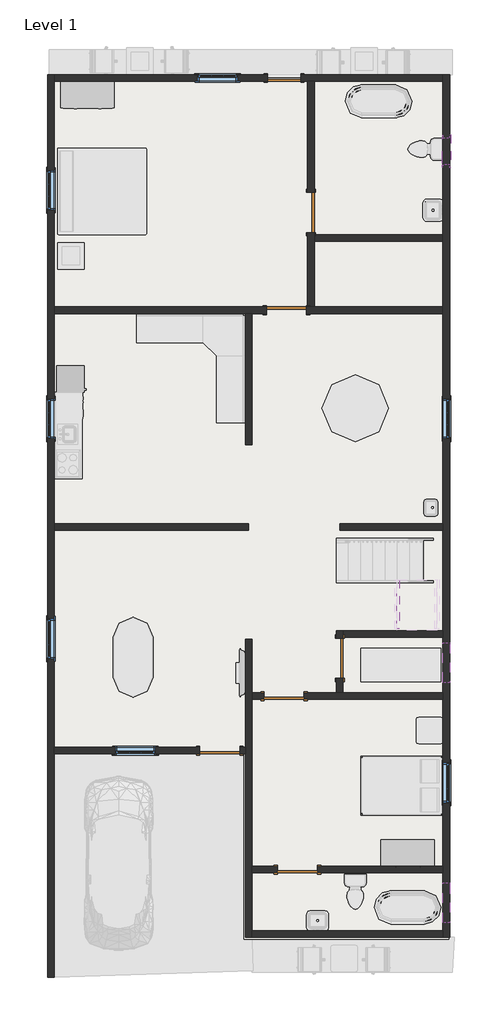
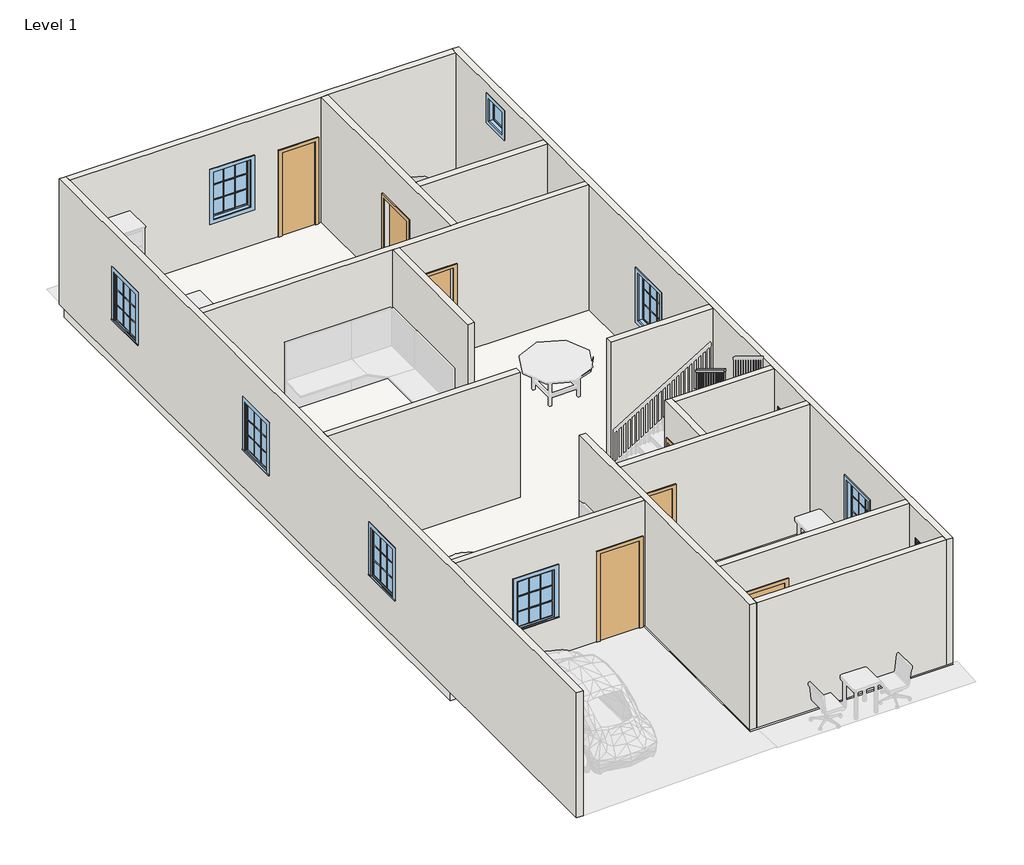
# One storey, part 1 of 2: 16 walls, 10 windows, 7 doors, 1 railing, 1 slab.
"""IFC4 building model written with IfcOpenShell, lengths in millimetres."""

from ifc_helpers import new_model, si_unit, frame, origin, origin_with_axes, place, context, project, spatial, polyline, outline, extrude, faceted_brep, transform, mapped, element, save
from components import door_255cab33, door_16372e1c, door_686f89d2, window_5c190c7e, window_fef7ae9c, window_3d781103

model = new_model("IFC4")

# Units and contexts
model_context = context("Model", 3, world=origin())
ifc_project = project(units=[si_unit("LENGTHUNIT", "METRE", prefix="MILLI")], contexts=[model_context])

# Site, building, storey
site = spatial("IfcSite", under=ifc_project)
building = spatial("IfcBuilding", under=site)
storey = spatial("IfcBuildingStorey", under=building, Name="Level 1", Elevation=0.0)

# Doors
placement = place(None, origin())
door_shape = door_255cab33(model_context)
element("IfcDoor", 1, ObjectType="Single-Flush : 30\" x 80\"", at=placement, inside=storey, context=model_context, shape_type="MappedRepresentation", body=[
    mapped(door_shape, transform((-7141.5873398, 12389.5549175, 0.0), x_axis=(1.0, 0.0, 0.0), y_axis=(0.0, 1.0, 0.0), z_axis=(0.0, 0.0, 1.0))),
])
door_2_shape = door_16372e1c(model_context)
element("IfcDoor", 2, ObjectType="Single-Flush : 36\" x 84\"", at=placement, inside=storey, context=model_context, shape_type="MappedRepresentation", body=[
    mapped(door_2_shape, transform((-7090.7873398, 7080.9549175, 0.0), x_axis=(1.0, 0.0, 0.0), y_axis=(0.0, 1.0, 0.0), z_axis=(0.0, 0.0, 1.0))),
])
element("IfcDoor", 3, ObjectType="Single-Flush : 36\" x 84\"", at=placement, inside=storey, context=model_context, shape_type="MappedRepresentation", body=[
    mapped(door_2_shape, transform((-6531.9873398, 9316.1549175, 0.0), x_axis=(0.0, -1.0, 0.0), y_axis=(1.0, 0.0, 0.0), z_axis=(0.0, 0.0, 1.0))),
])
element("IfcDoor", 4, ObjectType="Single-Flush : 36\" x 84\"", at=placement, inside=storey, context=model_context, shape_type="MappedRepresentation", body=[
    mapped(door_2_shape, transform((-7141.5873398, -1732.8450825, 0.0), x_axis=(-1.0, 0.0, 0.0), y_axis=(0.0, -1.0, 0.0), z_axis=(0.0, 0.0, 1.0))),
])
element("IfcDoor", 5, ObjectType="Single-Flush : 36\" x 84\"", at=placement, inside=storey, context=model_context, shape_type="MappedRepresentation", body=[
    mapped(door_2_shape, transform((-6836.7873398, -5695.2450825, 0.0), x_axis=(-1.0, 0.0, 0.0), y_axis=(0.0, -1.0, 0.0), z_axis=(0.0, 0.0, 1.0))),
])
door_3_shape = door_686f89d2(model_context)
element("IfcDoor", 6, ObjectType="Single-Flush : 36\" x 84\"", at=placement, inside=storey, context=model_context, shape_type="MappedRepresentation", body=[
    mapped(door_3_shape, transform((-8614.7873398, -2977.4450825, 0.0), x_axis=(1.0, 0.0, 0.0), y_axis=(0.0, 1.0, 0.0), z_axis=(0.0, 0.0, 1.0))),
])
element("IfcDoor", 7, ObjectType="Single-Flush : 36\" x 84\"", at=placement, inside=storey, context=model_context, shape_type="MappedRepresentation", body=[
    mapped(door_3_shape, transform((-5871.5873398, -869.2450825, 0.0), x_axis=(0.0, 1.0, 0.0), y_axis=(-1.0, 0.0, 0.0), z_axis=(0.0, 0.0, 1.0))),
])

# Railing
element("IfcRailing", 8, ObjectType="Handrail - Rectangular", at=placement, inside=storey, context=model_context, shape_type="SweptSolid", body=[
    extrude(outline(polyline([(923.5061342, 2607.7333333), (923.5061342, 2548.3318731), (-194.0938658, 3225.6652064), (-194.0938658, 3285.0666667), (923.5061342, 2607.7333333)])), frame((-4563.8448749, 0.0, 0.0), z_axis=(1.0, 0.0, 0.0), x_axis=(0.0, 1.0, 0.0)), (0.0, 0.0, 1.0), 50.8),
    extrude(outline(polyline([(831.4311342, 2604.1349034), (831.4311342, 1693.3333333), (812.3811342, 1693.3333333), (812.3811342, 2615.6803579), (831.4311342, 2604.1349034)])), frame((-4547.9698749, 0.0, 0.0), z_axis=(1.0, 0.0, 0.0), x_axis=(0.0, 1.0, 0.0)), (0.0, 0.0, 1.0), 19.05),
    extrude(outline(polyline([(729.8311342, 2665.710661), (729.8311342, 1693.3333333), (710.7811342, 1693.3333333), (710.7811342, 2677.2561155), (729.8311342, 2665.710661)])), frame((-4547.9698749, 0.0, 0.0), z_axis=(1.0, 0.0, 0.0), x_axis=(0.0, 1.0, 0.0)), (0.0, 0.0, 1.0), 19.05),
    extrude(outline(polyline([(628.2311342, 2727.2864185), (628.2311342, 1862.6666667), (609.1811342, 1862.6666667), (609.1811342, 2738.8318731), (628.2311342, 2727.2864185)])), frame((-4547.9698749, 0.0, 0.0), z_axis=(1.0, 0.0, 0.0), x_axis=(0.0, 1.0, 0.0)), (0.0, 0.0, 1.0), 19.05),
    extrude(outline(polyline([(526.6311342, 2788.8621761), (526.6311342, 1862.6666667), (507.5811342, 1862.6666667), (507.5811342, 2800.4076307), (526.6311342, 2788.8621761)])), frame((-4547.9698749, 0.0, 0.0), z_axis=(1.0, 0.0, 0.0), x_axis=(0.0, 1.0, 0.0)), (0.0, 0.0, 1.0), 19.05),
    extrude(outline(polyline([(425.0311342, 2850.4379337), (425.0311342, 1862.6666667), (405.9811342, 1862.6666667), (405.9811342, 2861.9833882), (425.0311342, 2850.4379337)])), frame((-4547.9698749, 0.0, 0.0), z_axis=(1.0, 0.0, 0.0), x_axis=(0.0, 1.0, 0.0)), (0.0, 0.0, 1.0), 19.05),
    extrude(outline(polyline([(323.4311342, 2912.0136913), (323.4311342, 2032.0), (304.3811342, 2032.0), (304.3811342, 2923.5591458), (323.4311342, 2912.0136913)])), frame((-4547.9698749, 0.0, 0.0), z_axis=(1.0, 0.0, 0.0), x_axis=(0.0, 1.0, 0.0)), (0.0, 0.0, 1.0), 19.05),
    extrude(outline(polyline([(221.8311342, 2973.5894488), (221.8311342, 2032.0), (202.7811342, 2032.0), (202.7811342, 2985.1349034), (221.8311342, 2973.5894488)])), frame((-4547.9698749, 0.0, 0.0), z_axis=(1.0, 0.0, 0.0), x_axis=(0.0, 1.0, 0.0)), (0.0, 0.0, 1.0), 19.05),
    extrude(outline(polyline([(120.2311342, 3035.1652064), (120.2311342, 2032.0), (101.1811342, 2032.0), (101.1811342, 3046.710661), (120.2311342, 3035.1652064)])), frame((-4547.9698749, 0.0, 0.0), z_axis=(1.0, 0.0, 0.0), x_axis=(0.0, 1.0, 0.0)), (0.0, 0.0, 1.0), 19.05),
    extrude(outline(polyline([(18.6311342, 3096.740964), (18.6311342, 2201.3333333), (-0.4188658, 2201.3333333), (-0.4188658, 3108.2864185), (18.6311342, 3096.740964)])), frame((-4547.9698749, 0.0, 0.0), z_axis=(1.0, 0.0, 0.0), x_axis=(0.0, 1.0, 0.0)), (0.0, 0.0, 1.0), 19.05),
    extrude(outline(polyline([(-82.9688658, 3158.3167216), (-82.9688658, 2201.3333333), (-102.0188658, 2201.3333333), (-102.0188658, 3169.8621761), (-82.9688658, 3158.3167216)])), frame((-4547.9698749, 0.0, 0.0), z_axis=(1.0, 0.0, 0.0), x_axis=(0.0, 1.0, 0.0)), (0.0, 0.0, 1.0), 19.05),
    extrude(outline(polyline([(923.5061342, 2548.3318731), (923.5061342, 1693.3333333), (904.4561342, 1693.3333333), (904.4561342, 2559.8773276), (923.5061342, 2548.3318731)])), frame((-4547.9698749, 0.0, 0.0), z_axis=(1.0, 0.0, 0.0), x_axis=(0.0, 1.0, 0.0)), (0.0, 0.0, 1.0), 19.05),
    extrude(outline(polyline([(-175.0438658, 3214.1197519), (-175.0438658, 2201.3333333), (-194.0938658, 2201.3333333), (-194.0938658, 3225.6652064), (-175.0438658, 3214.1197519)])), frame((-4547.9698749, 0.0, 0.0), z_axis=(1.0, 0.0, 0.0), x_axis=(0.0, 1.0, 0.0)), (0.0, 0.0, 1.0), 19.05),
])

# Slab
element("IfcSlab", 9, ObjectType="Generic - 12\"", at=placement, inside=storey, context=model_context, shape_type="SweptSolid", body=[
    extrude(outline(polyline([(-3376.8980823, 12389.5549175), (-3376.8980823, -7290.3890671), (-8055.9873398, -7290.3890671), (-8055.9873398, -2997.7890671), (-12475.5873398, -2997.7890671), (-12475.5873398, 12389.5549175), (-3376.8980823, 12389.5549175)])), frame((0.0, 0.0, -304.8), z_axis=(0.0, 0.0, 1.0), x_axis=(1.0, 0.0, 0.0)), (0.0, 0.0, 1.0), 304.8),
])

# Walls
element("IfcWall", 10, ObjectType="Generic - 8\"", at=placement, inside=storey, context=model_context, shape_type="Brep", body=[
    faceted_brep([(-12399.3873398, -8159.0450825, 0.0), (-12399.3873398, -3053.6450825, 0.0), (-12399.3873398, -2901.2450825, 0.0), (-12399.3873398, 2051.7549175, 0.0), (-12399.3873398, 2204.1549175, 0.0), (-12399.3873398, 7004.7549175, 0.0), (-12399.3873398, 7157.1549175, 0.0), (-12399.3873398, 12313.3549175, 0.0), (-12399.3873398, 12465.7549175, 0.0), (-12399.3873398, 12465.7549175, 3048.0), (-12399.3873398, 12313.3549175, 3048.0), (-12399.3873398, 7157.1549175, 3048.0), (-12399.3873398, 7004.7549175, 3048.0), (-12399.3873398, 2204.1549175, 3048.0), (-12399.3873398, 2051.7549175, 3048.0), (-12399.3873398, -2901.2450825, 3048.0), (-12399.3873398, -3053.6450825, 3048.0), (-12399.3873398, -8159.0450825, 3048.0), (-12399.3873398, 5061.6549175, 2133.6), (-12399.3873398, 5061.6549175, 914.4), (-12399.3873398, 4147.2549175, 914.4), (-12399.3873398, 4147.2549175, 2133.6), (-12399.3873398, 32.4549175, 2133.6), (-12399.3873398, 32.4549175, 914.4), (-12399.3873398, -881.9450825, 914.4), (-12399.3873398, -881.9450825, 2133.6), (-12399.3873398, 10281.3549175, 2133.6), (-12399.3873398, 10281.3549175, 914.4), (-12399.3873398, 9366.9549175, 914.4), (-12399.3873398, 9366.9549175, 2133.6), (-12551.7873398, -8159.0450825, 0.0), (-12551.7873398, -8159.0450825, 3048.0), (-12551.7873398, 12465.7549175, 3048.0), (-12551.7873398, 12465.7549175, 0.0), (-12551.7873398, 5061.6549175, 2133.6), (-12551.7873398, 4147.2549175, 2133.6), (-12551.7873398, 4147.2549175, 914.4), (-12551.7873398, 5061.6549175, 914.4), (-12551.7873398, 32.4549175, 2133.6), (-12551.7873398, -881.9450825, 2133.6), (-12551.7873398, -881.9450825, 914.4), (-12551.7873398, 32.4549175, 914.4), (-12551.7873398, 10281.3549175, 2133.6), (-12551.7873398, 9366.9549175, 2133.6), (-12551.7873398, 9366.9549175, 914.4), (-12551.7873398, 10281.3549175, 914.4)], [[[0, 1, 2, 3, 4, 5, 6, 7, 8, 9, 10, 11, 12, 13, 14, 15, 16, 17], [18, 19, 20, 21], [22, 23, 24, 25], [26, 27, 28, 29]], [[30, 31, 32, 33], [34, 35, 36, 37], [38, 39, 40, 41], [42, 43, 44, 45]], [[8, 7, 6, 5, 4, 3, 2, 1, 0, 30, 33]], [[17, 16, 15, 14, 13, 12, 11, 10, 9, 32, 31]], [[0, 17, 31, 30]], [[9, 8, 33, 32]], [[19, 18, 34, 37]], [[20, 19, 37, 36]], [[21, 20, 36, 35]], [[18, 21, 35, 34]], [[23, 22, 38, 41]], [[24, 23, 41, 40]], [[25, 24, 40, 39]], [[22, 25, 39, 38]], [[27, 26, 42, 45]], [[28, 27, 45, 44]], [[29, 28, 44, 43]], [[26, 29, 43, 42]]]),
])
element("IfcWall", 11, ObjectType="Generic - 8\"", at=placement, inside=storey, context=model_context, shape_type="Brep", body=[
    faceted_brep([(-6760.5873398, 12313.3549175, 2032.0), (-6760.5873398, 12313.3549175, 0.0), (-6608.1873398, 12313.3549175, 0.0), (-6455.7873398, 12313.3549175, 0.0), (-3509.3873398, 12313.3549175, 0.0), (-3509.3873398, 12313.3549175, 3048.0), (-6455.7873398, 12313.3549175, 3048.0), (-6608.1873398, 12313.3549175, 3048.0), (-12399.3873398, 12313.3549175, 3048.0), (-12399.3873398, 12313.3549175, 0.0), (-7522.5873398, 12313.3549175, 0.0), (-7522.5873398, 12313.3549175, 2032.0), (-8208.3873398, 12313.3549175, 2133.6), (-8208.3873398, 12313.3549175, 914.4), (-9122.7873398, 12313.3549175, 914.4), (-9122.7873398, 12313.3549175, 2133.6), (-3509.3873398, 12465.7549175, 0.0), (-6760.5873398, 12465.7549175, 0.0), (-6760.5873398, 12465.7549175, 2032.0), (-7522.5873398, 12465.7549175, 2032.0), (-7522.5873398, 12465.7549175, 0.0), (-12399.3873398, 12465.7549175, 0.0), (-12399.3873398, 12465.7549175, 3048.0), (-3509.3873398, 12465.7549175, 3048.0), (-8208.3873398, 12465.7549175, 2133.6), (-9122.7873398, 12465.7549175, 2133.6), (-9122.7873398, 12465.7549175, 914.4), (-8208.3873398, 12465.7549175, 914.4)], [[[0, 1, 2, 3, 4, 5, 6, 7, 8, 9, 10, 11], [12, 13, 14, 15]], [[16, 17, 18, 19, 20, 21, 22, 23], [24, 25, 26, 27]], [[10, 9, 21, 20]], [[4, 3, 2, 1, 17, 16]], [[8, 7, 6, 5, 23, 22]], [[5, 4, 16, 23]], [[9, 8, 22, 21]], [[13, 12, 24, 27]], [[14, 13, 27, 26]], [[15, 14, 26, 25]], [[12, 15, 25, 24]], [[18, 17, 1, 0]], [[19, 18, 0, 11]], [[20, 19, 11, 10]]]),
])
element("IfcWall", 12, ObjectType="Generic - 8\"", at=placement, inside=storey, context=model_context, shape_type="Brep", body=[
    faceted_brep([(-6608.1873398, 8858.9549175, 2133.6), (-6608.1873398, 8858.9549175, 0.0), (-6608.1873398, 7157.1549175, 0.0), (-6608.1873398, 7157.1549175, 3048.0), (-6608.1873398, 12313.3549175, 3048.0), (-6608.1873398, 12313.3549175, 0.0), (-6608.1873398, 9773.3549175, 0.0), (-6608.1873398, 9773.3549175, 2133.6), (-6455.7873398, 7157.1549175, 0.0), (-6455.7873398, 8655.7549175, 0.0), (-6455.7873398, 8808.1549175, 0.0), (-6455.7873398, 8858.9549175, 0.0), (-6455.7873398, 8858.9549175, 2133.6), (-6455.7873398, 9773.3549175, 2133.6), (-6455.7873398, 9773.3549175, 0.0), (-6455.7873398, 12313.3549175, 0.0), (-6455.7873398, 12313.3549175, 3048.0), (-6455.7873398, 8808.1549175, 3048.0), (-6455.7873398, 8655.7549175, 3048.0), (-6455.7873398, 7157.1549175, 3048.0)], [[[0, 1, 2, 3, 4, 5, 6, 7]], [[8, 9, 10, 11, 12, 13, 14, 15, 16, 17, 18, 19]], [[6, 5, 15, 14]], [[2, 1, 11, 10, 9, 8]], [[4, 3, 19, 18, 17, 16]], [[5, 4, 16, 15]], [[3, 2, 8, 19]], [[12, 11, 1, 0]], [[13, 12, 0, 7]], [[14, 13, 7, 6]]]),
])
element("IfcWall", 13, ObjectType="Generic - 8\"", at=placement, inside=storey, context=model_context, shape_type="Brep", body=[
    faceted_brep([(-6633.5873398, 7004.7549175, 2133.6), (-6633.5873398, 7004.7549175, 0.0), (-3509.3873398, 7004.7549175, 0.0), (-3509.3873398, 7004.7549175, 3048.0), (-7878.1873398, 7004.7549175, 3048.0), (-8030.5873398, 7004.7549175, 3048.0), (-12399.3873398, 7004.7549175, 3048.0), (-12399.3873398, 7004.7549175, 0.0), (-8030.5873398, 7004.7549175, 0.0), (-7878.1873398, 7004.7549175, 0.0), (-7547.9873398, 7004.7549175, 0.0), (-7547.9873398, 7004.7549175, 2133.6), (-3509.3873398, 7157.1549175, 0.0), (-6455.7873398, 7157.1549175, 0.0), (-6608.1873398, 7157.1549175, 0.0), (-6633.5873398, 7157.1549175, 0.0), (-6633.5873398, 7157.1549175, 2133.6), (-7547.9873398, 7157.1549175, 2133.6), (-7547.9873398, 7157.1549175, 0.0), (-12399.3873398, 7157.1549175, 0.0), (-12399.3873398, 7157.1549175, 3048.0), (-6608.1873398, 7157.1549175, 3048.0), (-6455.7873398, 7157.1549175, 3048.0), (-3509.3873398, 7157.1549175, 3048.0)], [[[0, 1, 2, 3, 4, 5, 6, 7, 8, 9, 10, 11]], [[12, 13, 14, 15, 16, 17, 18, 19, 20, 21, 22, 23]], [[2, 1, 15, 14, 13, 12]], [[10, 9, 8, 7, 19, 18]], [[6, 5, 4, 3, 23, 22, 21, 20]], [[3, 2, 12, 23]], [[7, 6, 20, 19]], [[16, 15, 1, 0]], [[17, 16, 0, 11]], [[18, 17, 11, 10]]]),
])
element("IfcWall", 14, ObjectType="Generic - 8\"", at=placement, inside=storey, context=model_context, shape_type="SweptSolid", body=[
    extrude(outline(polyline([(-8030.5873398, 4007.5549175), (-8030.5873398, 7004.7549175), (-7878.1873398, 7004.7549175), (-7878.1873398, 4007.5549175), (-8030.5873398, 4007.5549175)])), origin_with_axes(), (0.0, 0.0, 1.0), 3048.0),
])
element("IfcWall", 15, ObjectType="Generic - 8\"", at=placement, inside=storey, context=model_context, shape_type="SweptSolid", body=[
    extrude(outline(polyline([(-12399.3873398, 2204.1549175), (-7954.3873398, 2204.1549175), (-7954.3873398, 2051.7549175), (-12399.3873398, 2051.7549175), (-12399.3873398, 2204.1549175)])), origin_with_axes(), (0.0, 0.0, 1.0), 3048.0),
])
element("IfcWall", 16, ObjectType="Generic - 8\"", at=placement, inside=storey, context=model_context, shape_type="SweptSolid", body=[
    extrude(outline(polyline([(2133.6, -8157.5873398), (0.0, -8157.5873398), (0.0, -8030.5873398), (3048.0, -8030.5873398), (3048.0, -12399.3873398), (0.0, -12399.3873398), (0.0, -9071.9873398), (2133.6, -9071.9873398), (2133.6, -8157.5873398)]), holes=[polyline([(2133.6, -11002.3873398), (2133.6, -10087.9873398), (914.4, -10087.9873398), (914.4, -11002.3873398), (2133.6, -11002.3873398)])]), frame((0.0, -3053.6450825, 0.0), z_axis=(0.0, 1.0, 0.0), x_axis=(0.0, 0.0, 1.0)), (0.0, 0.0, 1.0), 152.4),
])
element("IfcWall", 17, ObjectType="Generic - 8\"", at=placement, inside=storey, context=model_context, shape_type="Brep", body=[
    faceted_brep([(-7878.1873398, -1809.0450825, 0.0), (-7598.7873398, -1809.0450825, 0.0), (-7598.7873398, -1809.0450825, 2133.6), (-6684.3873398, -1809.0450825, 2133.6), (-6684.3873398, -1809.0450825, 0.0), (-3509.3873398, -1809.0450825, 0.0), (-3509.3873398, -1809.0450825, 3048.0), (-7878.1873398, -1809.0450825, 3048.0), (-7598.7873398, -1656.6450825, 2133.6), (-7598.7873398, -1656.6450825, 0.0), (-7878.1873398, -1656.6450825, 0.0), (-7878.1873398, -1656.6450825, 3048.0), (-5947.7873398, -1656.6450825, 3048.0), (-5795.3873398, -1656.6450825, 3048.0), (-3509.3873398, -1656.6450825, 3048.0), (-3509.3873398, -1656.6450825, 0.0), (-5795.3873398, -1656.6450825, 0.0), (-5947.7873398, -1656.6450825, 0.0), (-6684.3873398, -1656.6450825, 0.0), (-6684.3873398, -1656.6450825, 2133.6)], [[[0, 1, 2, 3, 4, 5, 6, 7]], [[8, 9, 10, 11, 12, 13, 14, 15, 16, 17, 18, 19]], [[10, 9, 1, 0]], [[18, 17, 16, 15, 5, 4]], [[7, 6, 14, 13, 12, 11]], [[6, 5, 15, 14]], [[0, 7, 11, 10]], [[2, 1, 9, 8]], [[3, 2, 8, 19]], [[4, 3, 19, 18]]]),
])
element("IfcWall", 18, ObjectType="Generic - 8\"", at=placement, inside=storey, context=model_context, shape_type="SweptSolid", body=[
    extrude(outline(polyline([(-3509.3873398, -7244.6450825), (-7878.1873398, -7244.6450825), (-7878.1873398, -7092.2450825), (-3509.3873398, -7092.2450825), (-3509.3873398, -7244.6450825)])), origin_with_axes(), (0.0, 0.0, 1.0), 3048.0),
])
element("IfcWall", 19, ObjectType="Generic - 8\"", at=placement, inside=storey, context=model_context, shape_type="SweptSolid", body=[
    extrude(outline(polyline([(0.0, -7878.1873398), (0.0, -7293.9873398), (2133.6, -7293.9873398), (2133.6, -6379.5873398), (0.0, -6379.5873398), (0.0, -3509.3873398), (3048.0, -3509.3873398), (3048.0, -7878.1873398), (0.0, -7878.1873398)])), frame((0.0, -5771.4450825, 0.0), z_axis=(0.0, 1.0, 0.0), x_axis=(0.0, 0.0, 1.0)), (0.0, 0.0, 1.0), 152.4),
])
element("IfcWall", 20, ObjectType="Generic - 8\"", at=placement, inside=storey, context=model_context, shape_type="Brep", body=[
    faceted_brep([(-5795.3873398, -412.0450825, 2133.6), (-5795.3873398, -412.0450825, 0.0), (-5795.3873398, -386.6450825, 0.0), (-5795.3873398, -234.2450825, 0.0), (-5795.3873398, -234.2450825, 3048.0), (-5795.3873398, -386.6450825, 3048.0), (-5795.3873398, -1656.6450825, 3048.0), (-5795.3873398, -1656.6450825, 0.0), (-5795.3873398, -1326.4450825, 0.0), (-5795.3873398, -1326.4450825, 2133.6), (-5947.7873398, -234.2450825, 0.0), (-5947.7873398, -412.0450825, 0.0), (-5947.7873398, -412.0450825, 2133.6), (-5947.7873398, -1326.4450825, 2133.6), (-5947.7873398, -1326.4450825, 0.0), (-5947.7873398, -1656.6450825, 0.0), (-5947.7873398, -1656.6450825, 3048.0), (-5947.7873398, -234.2450825, 3048.0)], [[[0, 1, 2, 3, 4, 5, 6, 7, 8, 9]], [[10, 11, 12, 13, 14, 15, 16, 17]], [[8, 7, 15, 14]], [[3, 2, 1, 11, 10]], [[6, 5, 4, 17, 16]], [[7, 6, 16, 15]], [[4, 3, 10, 17]], [[12, 11, 1, 0]], [[13, 12, 0, 9]], [[14, 13, 9, 8]]]),
])
element("IfcWall", 21, ObjectType="Generic - 8\"", at=placement, inside=storey, context=model_context, shape_type="SweptSolid", body=[
    extrude(outline(polyline([(-3509.3873398, -386.6450825), (-5795.3873398, -386.6450825), (-5795.3873398, -234.2450825), (-3509.3873398, -234.2450825), (-3509.3873398, -386.6450825)])), origin_with_axes(), (0.0, 0.0, 1.0), 3048.0),
])
element("IfcWall", 22, ObjectType="Generic - 8\"", at=placement, inside=storey, context=model_context, shape_type="SweptSolid", body=[
    extrude(outline(polyline([(-3509.3873398, 2051.7549175), (-5871.5873398, 2051.7549175), (-5871.5873398, 2204.1549175), (-3509.3873398, 2204.1549175), (-3509.3873398, 2051.7549175)])), origin_with_axes(), (0.0, 0.0, 1.0), 3048.0),
])
element("IfcWall", 23, ObjectType="Generic - 8\"", at=placement, inside=storey, context=model_context, shape_type="SweptSolid", body=[
    extrude(outline(polyline([(-3509.3873398, 8655.7549175), (-6455.7873398, 8655.7549175), (-6455.7873398, 8808.1549175), (-3509.3873398, 8808.1549175), (-3509.3873398, 8655.7549175)])), origin_with_axes(), (0.0, 0.0, 1.0), 3048.0),
])
element("IfcWall", 24, ObjectType="Generic - 8\"", at=placement, inside=storey, context=model_context, shape_type="Brep", body=[
    faceted_brep([(-8030.5873398, -437.4450825, 0.0), (-8030.5873398, -2901.2450825, 0.0), (-8030.5873398, -3053.6450825, 0.0), (-8030.5873398, -7244.6450825, 0.0), (-8030.5873398, -7244.6450825, 3048.0), (-8030.5873398, -3053.6450825, 3048.0), (-8030.5873398, -2901.2450825, 3048.0), (-8030.5873398, -437.4450825, 3048.0), (-7878.1873398, -437.4450825, 0.0), (-7878.1873398, -437.4450825, 3048.0), (-7878.1873398, -1656.6450825, 3048.0), (-7878.1873398, -1809.0450825, 3048.0), (-7878.1873398, -5619.0450825, 3048.0), (-7878.1873398, -5771.4450825, 3048.0), (-7878.1873398, -7092.2450825, 3048.0), (-7878.1873398, -7244.6450825, 3048.0), (-7878.1873398, -7244.6450825, 0.0), (-7878.1873398, -7092.2450825, 0.0), (-7878.1873398, -5771.4450825, 0.0), (-7878.1873398, -5619.0450825, 0.0), (-7878.1873398, -1809.0450825, 0.0), (-7878.1873398, -1656.6450825, 0.0)], [[[0, 1, 2, 3, 4, 5, 6, 7]], [[8, 9, 10, 11, 12, 13, 14, 15, 16, 17, 18, 19, 20, 21]], [[3, 2, 1, 0, 8, 21, 20, 19, 18, 17, 16]], [[7, 6, 5, 4, 15, 14, 13, 12, 11, 10, 9]], [[0, 7, 9, 8]], [[4, 3, 16, 15]]]),
])
element("IfcWall", 25, ObjectType="Generic - 8\"", at=placement, inside=storey, context=model_context, shape_type="Brep", body=[
    faceted_brep([(-3509.3873398, 12465.7549175, 0.0), (-3509.3873398, 12313.3549175, 0.0), (-3509.3873398, 8808.1549175, 0.0), (-3509.3873398, 8655.7549175, 0.0), (-3509.3873398, 7157.1549175, 0.0), (-3509.3873398, 7004.7549175, 0.0), (-3509.3873398, 2204.1549175, 0.0), (-3509.3873398, 2051.7549175, 0.0), (-3509.3873398, -234.2450825, 0.0), (-3509.3873398, -386.6450825, 0.0), (-3509.3873398, -1656.6450825, 0.0), (-3509.3873398, -1809.0450825, 0.0), (-3509.3873398, -5619.0450825, 0.0), (-3509.3873398, -5771.4450825, 0.0), (-3509.3873398, -7092.2450825, 0.0), (-3509.3873398, -7244.6450825, 0.0), (-3509.3873398, -7244.6450825, 3048.0), (-3509.3873398, -7092.2450825, 3048.0), (-3509.3873398, -5771.4450825, 3048.0), (-3509.3873398, -5619.0450825, 3048.0), (-3509.3873398, -1809.0450825, 3048.0), (-3509.3873398, -1656.6450825, 3048.0), (-3509.3873398, -386.6450825, 3048.0), (-3509.3873398, -234.2450825, 3048.0), (-3509.3873398, 2051.7549175, 3048.0), (-3509.3873398, 2204.1549175, 3048.0), (-3509.3873398, 7004.7549175, 3048.0), (-3509.3873398, 7157.1549175, 3048.0), (-3509.3873398, 8655.7549175, 3048.0), (-3509.3873398, 8808.1549175, 3048.0), (-3509.3873398, 12313.3549175, 3048.0), (-3509.3873398, 12465.7549175, 3048.0), (-3509.3873398, -4171.2450825, 2133.6), (-3509.3873398, -4171.2450825, 914.4), (-3509.3873398, -3256.8450825, 914.4), (-3509.3873398, -3256.8450825, 2133.6), (-3509.3873398, 4147.2549175, 2133.6), (-3509.3873398, 4147.2549175, 914.4), (-3509.3873398, 5061.6549175, 914.4), (-3509.3873398, 5061.6549175, 2133.6), (-3509.3873398, 10408.3549175, 2768.6), (-3509.3873398, 10408.3549175, 2159.0), (-3509.3873398, 11017.9549175, 2159.0), (-3509.3873398, 11017.9549175, 2768.6), (-3509.3873398, -6000.0450825, 2346.3107302), (-3509.3873398, -6914.4450825, 2346.3107302), (-3509.3873398, -6914.4450825, 1736.7107302), (-3509.3873398, -6000.0450825, 1736.7107302), (-3509.3873398, -513.6450825, 2215.7397197), (-3509.3873398, -1428.0450825, 2215.7397197), (-3509.3873398, -1428.0450825, 1606.1397197), (-3509.3873398, -513.6450825, 1606.1397197), (-3356.9873398, 12465.7549175, 0.0), (-3356.9873398, 12465.7549175, 3048.0), (-3356.9873398, -7244.6450825, 3048.0), (-3356.9873398, -7244.6450825, 0.0), (-3356.9873398, -4171.2450825, 2133.6), (-3356.9873398, -3256.8450825, 2133.6), (-3356.9873398, -3256.8450825, 914.4), (-3356.9873398, -4171.2450825, 914.4), (-3356.9873398, 4147.2549175, 2133.6), (-3356.9873398, 5061.6549175, 2133.6), (-3356.9873398, 5061.6549175, 914.4), (-3356.9873398, 4147.2549175, 914.4), (-3356.9873398, 10408.3549175, 2768.6), (-3356.9873398, 11017.9549175, 2768.6), (-3356.9873398, 11017.9549175, 2159.0), (-3356.9873398, 10408.3549175, 2159.0), (-3356.9873398, -6000.0450825, 2346.3107302), (-3356.9873398, -6000.0450825, 1736.7107302), (-3356.9873398, -6914.4450825, 1736.7107302), (-3356.9873398, -6914.4450825, 2346.3107302), (-3356.9873398, -513.6450825, 2215.7397197), (-3356.9873398, -513.6450825, 1606.1397197), (-3356.9873398, -1428.0450825, 1606.1397197), (-3356.9873398, -1428.0450825, 2215.7397197)], [[[0, 1, 2, 3, 4, 5, 6, 7, 8, 9, 10, 11, 12, 13, 14, 15, 16, 17, 18, 19, 20, 21, 22, 23, 24, 25, 26, 27, 28, 29, 30, 31], [32, 33, 34, 35], [36, 37, 38, 39], [40, 41, 42, 43], [44, 45, 46, 47], [48, 49, 50, 51]], [[52, 53, 54, 55], [56, 57, 58, 59], [60, 61, 62, 63], [64, 65, 66, 67], [68, 69, 70, 71], [72, 73, 74, 75]], [[15, 14, 13, 12, 11, 10, 9, 8, 7, 6, 5, 4, 3, 2, 1, 0, 52, 55]], [[31, 30, 29, 28, 27, 26, 25, 24, 23, 22, 21, 20, 19, 18, 17, 16, 54, 53]], [[16, 15, 55, 54]], [[0, 31, 53, 52]], [[33, 32, 56, 59]], [[34, 33, 59, 58]], [[35, 34, 58, 57]], [[32, 35, 57, 56]], [[37, 36, 60, 63]], [[38, 37, 63, 62]], [[39, 38, 62, 61]], [[36, 39, 61, 60]], [[41, 40, 64, 67]], [[42, 41, 67, 66]], [[43, 42, 66, 65]], [[40, 43, 65, 64]], [[69, 68, 44, 47]], [[70, 69, 47, 46]], [[71, 70, 46, 45]], [[68, 71, 45, 44]], [[73, 72, 48, 51]], [[74, 73, 51, 50]], [[75, 74, 50, 49]], [[72, 75, 49, 48]]]),
])

# Windows
window_shape = window_5c190c7e(model_context)
element("IfcWindow", 26, ObjectType="Casement 3x3 with Trim : 36\" x 48\"", at=placement, inside=storey, context=model_context, shape_type="MappedRepresentation", body=[
    mapped(window_shape, transform((-8665.5873398, 12389.5549175, 0.0), x_axis=(1.0, 0.0, 0.0), y_axis=(0.0, 1.0, 0.0), z_axis=(0.0, 0.0, 1.0))),
])
element("IfcWindow", 27, ObjectType="Casement 3x3 with Trim : 36\" x 48\"", at=placement, inside=storey, context=model_context, shape_type="MappedRepresentation", body=[
    mapped(window_shape, transform((-12475.5873398, 4604.4549175, 0.0), x_axis=(0.0, 1.0, 0.0), y_axis=(-1.0, 0.0, 0.0), z_axis=(0.0, 0.0, 1.0))),
])
element("IfcWindow", 28, ObjectType="Casement 3x3 with Trim : 36\" x 48\"", at=placement, inside=storey, context=model_context, shape_type="MappedRepresentation", body=[
    mapped(window_shape, transform((-12475.5873398, -424.7450825, 0.0), x_axis=(0.0, 1.0, 0.0), y_axis=(-1.0, 0.0, 0.0), z_axis=(0.0, 0.0, 1.0))),
])
element("IfcWindow", 29, ObjectType="Casement 3x3 with Trim : 36\" x 48\"", at=placement, inside=storey, context=model_context, shape_type="MappedRepresentation", body=[
    mapped(window_shape, transform((-10545.1873398, -2977.4450825, 0.0), x_axis=(-1.0, 0.0, 0.0), y_axis=(0.0, -1.0, 0.0), z_axis=(0.0, 0.0, 1.0))),
])
element("IfcWindow", 30, ObjectType="Casement 3x3 with Trim : 36\" x 48\"", at=placement, inside=storey, context=model_context, shape_type="MappedRepresentation", body=[
    mapped(window_shape, transform((-3433.1873398, -3714.0450825, 0.0), x_axis=(0.0, -1.0, 0.0), y_axis=(1.0, 0.0, 0.0), z_axis=(0.0, 0.0, 1.0))),
])
element("IfcWindow", 31, ObjectType="Casement 3x3 with Trim : 36\" x 48\"", at=placement, inside=storey, context=model_context, shape_type="MappedRepresentation", body=[
    mapped(window_shape, transform((-3433.1873398, 4604.4549175, 0.0), x_axis=(0.0, -1.0, 0.0), y_axis=(1.0, 0.0, 0.0), z_axis=(0.0, 0.0, 1.0))),
])
element("IfcWindow", 32, ObjectType="Casement 3x3 with Trim : 36\" x 48\"", at=placement, inside=storey, context=model_context, shape_type="MappedRepresentation", body=[
    mapped(window_shape, transform((-12475.5873398, 9824.1549175, 0.0), x_axis=(0.0, 1.0, 0.0), y_axis=(-1.0, 0.0, 0.0), z_axis=(0.0, 0.0, 1.0))),
])
window_2_shape = window_fef7ae9c(model_context)
element("IfcWindow", 33, ObjectType="Fixed : 36\" x 24\"", at=placement, inside=storey, context=model_context, shape_type="MappedRepresentation", body=[
    mapped(window_2_shape, transform((-3433.1873398, -6419.1450825, 822.3107302), x_axis=(0.0, 1.0, 0.0), y_axis=(-1.0, 0.0, 0.0), z_axis=(0.0, 0.0, 1.0))),
])
element("IfcWindow", 34, ObjectType="Fixed : 36\" x 24\"", at=placement, inside=storey, context=model_context, shape_type="MappedRepresentation", body=[
    mapped(window_2_shape, transform((-3433.1873398, -932.7450825, 691.7397197), x_axis=(0.0, 1.0, 0.0), y_axis=(-1.0, 0.0, 0.0), z_axis=(0.0, 0.0, 1.0))),
])
window_3_shape = window_3d781103(model_context)
element("IfcWindow", 35, ObjectType="Transom with Trim : 24\" x 24\"", at=placement, inside=storey, context=model_context, shape_type="MappedRepresentation", body=[
    mapped(window_3_shape, transform((-3433.1873398, 10675.0549175, 0.0), x_axis=(0.0, -1.0, 0.0), y_axis=(1.0, 0.0, 0.0), z_axis=(0.0, 0.0, 1.0))),
])

save(model, "model.ifc")

# Revit data of these elements
# Type "Single-Flush : 30\" x 80\""
#   Type Mark = "5"
#   Construction Type Id = "MDOOR"
#   Assembly Code = "C1020"
#   Analytic Construction = "Metal"
#   Thickness = 0' - 2"
#   Heat Transfer Coefficient (U) = 0.651978 BTU/(h·ft²·°F)
#   Height = 6' - 8"
#   Trim Projection Ext = 0' - 1"
#   Trim Projection Int = 0' - 1"
#   Trim Width = 0' - 3"
#   Width = 2' - 6"
#   Define Thermal Properties by = 1
#   Door Material = Door - Panel
#   Frame Material = Door - Frame
#   Visual Light Transmittance = 0
#   Solar Heat Gain Coefficient = 0
#   Function = (empty or 0)
#   Wall Closure = (empty or 0)
# Type "Single-Flush : 36\" x 84\""
#   Type Mark = "1"
#   Construction Type Id = "MDOOR"
#   Assembly Code = "C1020"
#   Analytic Construction = "Metal"
#   Thickness = 0' - 2"
#   Heat Transfer Coefficient (U) = 0.651978 BTU/(h·ft²·°F)
#   Height = 7' - 0"
#   Trim Projection Ext = 0' - 1"
#   Trim Projection Int = 0' - 1"
#   Trim Width = 0' - 3"
#   Width = 3' - 0"
#   Define Thermal Properties by = 1
#   Door Material = Door - Panel
#   Frame Material = Door - Frame
#   Visual Light Transmittance = 0
#   Solar Heat Gain Coefficient = 0
#   Function = (empty or 0)
#   Wall Closure = (empty or 0)
# Type "Handrail - Rectangular"
#   Assembly Code = "C2010400"
#   built-in parameter 1008612 = 0.0416667 (stored number, unit not read)
#   built-in parameter 1008611 = 0.0416667 (stored number, unit not read)
#   built-in parameter 1008609 = 0.333333 (stored number, unit not read)
#   built-in parameter 1008604 = 0.166667 (stored number, unit not read)
#   built-in parameter 1008603 = 0.166667 (stored number, unit not read)
#   Railing Height = 3' - 0"
#   built-in parameter 1008630 = 2
#   built-in parameter 1008610 = 2
#   built-in parameter 1008618 = Baluster - Square : 3/4"
# Type "Generic - 12\""
#   Assembly Code = "B1010"
#   Function = 0
#   Layers, outside or top first: 1' - 0" no material (function 1)
# Type "Generic - 8\""
#   Assembly Code = "B2010"
#   Layers, outside or top first: 0' - 6" "Brick, Common" (function 1)
# Type "Casement 3x3 with Trim : 36\" x 48\""
#   Type Mark = "10"
#   Construction Type Id = "GSP4R"
#   Assembly Code = "B2020100"
#   Analytic Construction = "1/8 in Pilkington single glazing"
#   Visual Light Transmittance = 0.9
#   Solar Heat Gain Coefficient = 0.78
#   Heat Transfer Coefficient (U) = 0.6496 BTU/(h·ft²·°F)
#   Height = 4' - 0"
#   Default Sill Height = 3' - 0"
#   Trim Projection - Ext. = 0' - 0 1/2"
#   Trim Projection - Int. = 0' - 0 3/4"
#   Trim Width - Exterior = 0' - 3 1/2"
#   Trim Width - Interior = 0' - 3 1/2"
#   Width = 3' - 0"
#   Window Inset = 0' - 0 3/4"
#   Define Thermal Properties by = 1
#   Glass Pane Material = Glass
#   Sash Material = Sash
#   Trim Exterior Material = Trim
#   Trim Interior Material = Trim
#   Wall Closure = (empty or 0)
# Type "Fixed : 36\" x 24\""
#   Type Mark = "8"
#   Construction Type Id = "GSP4R"
#   Assembly Code = "B2020100"
#   Analytic Construction = "1/8 in Pilkington single glazing"
#   Visual Light Transmittance = 0.9
#   Solar Heat Gain Coefficient = 0.78
#   Heat Transfer Coefficient (U) = 0.6496 BTU/(h·ft²·°F)
#   Height = 2' - 0"
#   Default Sill Height = 3' - 0"
#   Width = 3' - 0"
#   Window Inset = 0' - 0 3/4"
#   Define Thermal Properties by = 1
#   Glass Pane Material = Glass
#   Sash Material = Sash
#   Wall Closure = (empty or 0)
# Type "Transom with Trim : 24\" x 24\""
#   Type Mark = "13"
#   Construction Type Id = "GSP4R"
#   Assembly Code = "B2020100"
#   Analytic Construction = "1/8 in Pilkington single glazing"
#   Visual Light Transmittance = 0.9
#   Solar Heat Gain Coefficient = 0.78
#   Heat Transfer Coefficient (U) = 0.6496 BTU/(h·ft²·°F)
#   Height = 2' - 0"
#   Default Sill Height = 7' - 1"
#   Trim Projection - Ext. = 0' - 0 1/2"
#   Trim Projection - Int. = 0' - 0 3/4"
#   Trim Width - Exterior = 0' - 3 1/2"
#   Trim Width - Interior = 0' - 3 1/2"
#   Width = 2' - 0"
#   Window Inset = 0' - 0 3/4"
#   Define Thermal Properties by = 1
#   Glass Pane Material = Glass
#   Sash Material = Sash
#   Trim Exterior Material = Trim
#   Trim Interior Material = Trim
#   Wall Closure = (empty or 0)
# Element 1 (IfcDoor, "Single-Flush : 30\" x 80\"")
#   Phase Created = New Construction
#   Materials on its faces: "Door - Frame", "Door - Panel"
# Elements 2, 3, 4, 5, 6, 7 (IfcDoor, "Single-Flush : 36\" x 84\"")
#   Phase Created = New Construction
#   Materials on its faces: "Door - Frame", "Door - Panel"
# Element 8 (IfcRailing, "Handrail - Rectangular")
#   Phase Created = New Construction
# Element 9 (IfcSlab, "Generic - 12\"")
#   Height Offset From Level = 0' - 0"
#   Phase Created = New Construction
#   Materials on its faces: "Default Floor"
# Elements 10, 11, 12, 13, 14, 15, 16, 17, 18, 19, 20, 21, 22, 23, 24, 25 (IfcWall, "Generic - 8\"")
#   Top Offset = 0' - 0"
#   Base Offset = 0' - 0"
#   Unconnected Height = 10' - 0"
#   wall height = 10' - 0"
#   Phase Created = New Construction
#   Base Constraint = Level 1
#   Materials on its faces: "Brick, Common"
# Element 26 (IfcWindow, "Casement 3x3 with Trim : 36\" x 48\"")
#   Mark = "2"
#   Phase Created = New Construction
#   Materials on its faces: "Sash", "Glass", "Trim"
# Element 27 (IfcWindow, "Casement 3x3 with Trim : 36\" x 48\"")
#   Mark = "3"
#   Phase Created = New Construction
#   Materials on its faces: "Sash", "Glass", "Trim"
# Element 28 (IfcWindow, "Casement 3x3 with Trim : 36\" x 48\"")
#   Mark = "4"
#   Phase Created = New Construction
#   Materials on its faces: "Sash", "Glass", "Trim"
# Element 29 (IfcWindow, "Casement 3x3 with Trim : 36\" x 48\"")
#   Mark = "5"
#   Phase Created = New Construction
#   Materials on its faces: "Sash", "Glass", "Trim"
# Element 30 (IfcWindow, "Casement 3x3 with Trim : 36\" x 48\"")
#   Mark = "6"
#   Phase Created = New Construction
#   Materials on its faces: "Sash", "Glass", "Trim"
# Element 31 (IfcWindow, "Casement 3x3 with Trim : 36\" x 48\"")
#   Mark = "8"
#   Phase Created = New Construction
#   Materials on its faces: "Sash", "Glass", "Trim"
# Element 32 (IfcWindow, "Casement 3x3 with Trim : 36\" x 48\"")
#   Mark = "13"
#   Phase Created = New Construction
#   Materials on its faces: "Sash", "Glass", "Trim"
# Element 33 (IfcWindow, "Fixed : 36\" x 24\"")
#   Mark = "11"
#   Phase Created = New Construction
#   Materials on its faces: "Sash", "Glass"
# Element 34 (IfcWindow, "Fixed : 36\" x 24\"")
#   Mark = "12"
#   Phase Created = New Construction
#   Materials on its faces: "Sash", "Glass"
# Element 35 (IfcWindow, "Transom with Trim : 24\" x 24\"")
#   Mark = "10"
#   Phase Created = New Construction
#   Materials on its faces: "Sash", "Trim", "Glass"
# Materials
#   "Door - Panel": class "Wood", colour RGB 210 159 95, transparency 0
#   "Door - Frame": colour RGB 118 70 51, transparency 0
#   "Brick, Common": class "Masonry", colour RGB 170 98 104, transparency 0, Description = "Common brick", Cost = 0
#   "Glass": class "Glass", colour RGB 0 128 192, transparency 0.75, Description = "Soda Lime Glass", Cost = 0
#   "Sash": class "Wood", colour RGB 224 178 126, transparency 0
#   "Trim": class "Wood", colour RGB 224 178 126, transparency 0
#   "Default Floor": colour RGB 128 128 128, transparency 0
# Room at (-8353.229, 12510.178) mm, phase "New Construction", upper level "Level 1", upper offset 10' - 0", lower offset 0' - 0"
#   Number = "1"
#   Name = "REAR SPACE"
# Room at (-9459.993, 10505.303) mm, phase "New Construction", upper level "Level 1", upper offset 10' - 0", lower offset 0' - 0"
#   Number = "2"
#   Name = "BEDROOM"
# Room at (-4862.34, 10505.303) mm, phase "New Construction", upper level "Level 1", upper offset 10' - 0", lower offset 0' - 0"
#   Number = "3"
# Room at (-5069.297, 7760.812) mm, phase "New Construction", upper level "Level 1", upper offset 10' - 0", lower offset 0' - 0"
#   Number = "4"
#   Name = "DUCT"
# Room at (-10091.45, 4325.328) mm, phase "New Construction", upper level "Level 1", upper offset 10' - 0", lower offset 0' - 0"
#   Number = "5"
#   Name = "KITCHEN"
# Room at (-5069.297, 4325.328) mm, phase "New Construction", upper level "Level 1", upper offset 10' - 0", lower offset 0' - 0"
#   Number = "6"
#   Name = "DINING"
# Room at (-10091.45, -379.492) mm, phase "New Construction", upper level "Level 1", upper offset 10' - 0", lower offset 0' - 0"
#   Number = "7"
#   Name = "LIVING"
# Room at (-4572.6, 882.664) mm, phase "New Construction", upper level "Level 1", upper offset 10' - 0", lower offset 0' - 0"
#   Number = "8"
#   Name = "Room"
# Room at (-4572.6, -1152.131) mm, phase "New Construction", upper level "Level 1", upper offset 10' - 0", lower offset 0' - 0"
#   Number = "9"
#   Name = "Room"
# Room at (-10091.45, -5545.169) mm, phase "New Construction", upper level "Level 1", upper offset 10' - 0", lower offset 0' - 0"
#   Number = "10"
#   Name = "PARKING"
# Room at (-5886.707, -4283.014) mm, phase "New Construction", upper level "Level 1", upper offset 10' - 0", lower offset 0' - 0"
#   Number = "11"
#   Name = "BEDROOM"
# Room at (-5649.5, -6807.325) mm, phase "New Construction", upper level "Level 1", upper offset 10' - 0", lower offset 0' - 0"
#   Number = "12"
#   Name = "TOILET"
# Room at (-5649.5, -7716.526) mm, phase "New Construction", upper level "Level 1", upper offset 10' - 0", lower offset 0' - 0"
#   Number = "13"
#   Name = "LAWN"
